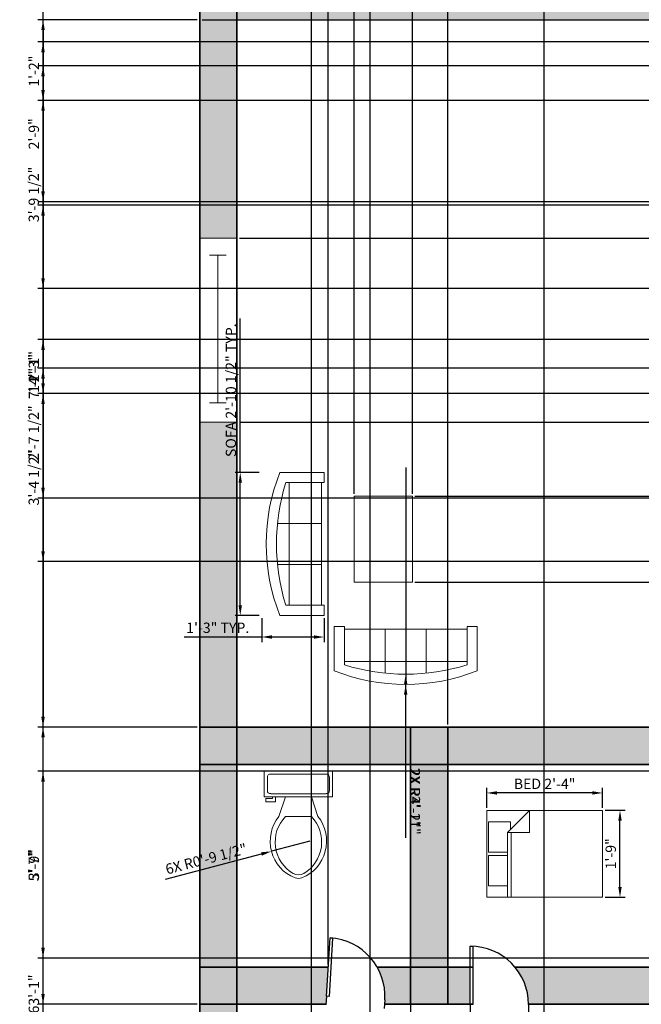
# Model space of a CAD drawing. Units: millimetres. Extents: x 2856 to 3283, y 634 to 1474.
# Tile 3 of 8: x 2856 to 3006, y 1050 to 1288. Entities that reach past the tile are written whole.
import ezdxf

# ---------------------------------------------------------------- set-up
doc = ezdxf.new("R2010")
doc.units = ezdxf.units.MM
for name, color, linetype, lineweight in [('A-ANNO-DIMS', 90, 'Continuous', 18), ('A-FLOR-FIXT', 140, 'Continuous', 18), ('A-WALL-PATT', 2, 'Continuous', 13), ('doors', 10, 'Continuous', 25), ('furniture', 140, 'Continuous', 18), ('walls', 50, 'Continuous', 35), ('windows', 30, 'Continuous', 18)]:
    doc.layers.add(name, color=color, linetype=linetype, lineweight=lineweight)
doc.styles.get("Standard").update_dxf_attribs({"font": 'arial.ttf'})
doc.dimstyles.new('ISO-25', dxfattribs={"dimtxt": 2.5, "dimasz": 2.5, "dimexe": 1.25, "dimexo": 0.625, "dimtad": 1, "dimdec": 0, "dimlunit": 3, "dimtxsty": 'Standard', "dimcen": 2.5, "dimadec": 0, "dimazin": 0, "dimtfac": 1, "dimtdec": 0, "dimtmove": 0, "dimatfit": 3, "dimfxl": 1, "dimarcsym": 0})

# ---------------------------------------------------------------- blocks, each defined once
blk = doc.blocks.new('*U3')
for p, q in [((0, 0), (0, -6)), ((40, 0), (40, -6))]:
    blk.add_line(p, q)
blk.add_lwpolyline([(0, 0), (0, 40), (1.75, 40), (1.75, 0)], close=True)
blk.add_arc((0, 0), 40, 0, 90)
blk = doc.blocks.new('*U5')
for p, q in [((0, 4), (0, 0)), ((36, 4), (36, 0)), ((0, 2), (36, 2))]:
    blk.add_line(p, q)
blk = doc.blocks.new('Bed - Queen')
for p, q in [((0, -80.00003), (0, 0)), ((0, 0), (59.99999, 0)), ((59.99999, 0), (59.99999, -80.00003)), ((7.99999, -1.2), (28.79998, -1.2)), ((7.99999, -14.4), (7.99999, -1.2)), ((28.79998, -1.2), (28.79998, -14.4)), ((31.19999, -1.2), (51.99999, -1.2)), ((31.19999, -14.4), (31.19999, -1.2)), ((51.99999, -1.2), (51.99999, -16.4)), ((0, -14.4), (44.8, -14.4)), ((44.8, -16.8), (0, -16.8)), ((59.99999, -29.6), (44.8, -14.4)), ((44.8, -14.4), (44.8, -29.6)), ((51.99999, -16.4), (46.79936, -16.4)), ((44.8, -29.6), (59.99999, -29.6)), ((59.99999, -80.00003), (0, -80.00003))]:
    blk.add_line(p, q)
blk = doc.blocks.new('Sofa - Roundback 7 ft.')
for p, q in [((-36.000027, -34), (-36.000027, -11.4696)), ((-12.00002, -32.4421), (-12.00003, -6.5971)), ((11.99997, -32.4421), (11.99998, -6.5971)), ((35.99998, -34), (35.99998, -11.4696)), ((-35.999844, -13.3819), (35.9998, -13.3819)), ((-36.000027, -32.4421), (35.99998, -32.4421))]:
    blk.add_line(p, q)
for points in [[(-36.000027, -34), (-42.000027, -34), (-42.000027, -8)], [(41.99998, -8), (41.99998, -34), (35.99998, -34)]]:
    blk.add_lwpolyline(points)
for centre, radius, start, end in [((0, -114.25), 114.25, 68.43141, 111.5686), ((-0.00001, -127.1968), 121.1968, 72.72033, 107.2797)]:
    blk.add_arc(centre, radius, start, end)
blk = doc.blocks.new('Toilet - top')
for p, q in [((9.5, -6), (9.5, -2)), ((-10, -8.5), (-8, -8.5)), ((-10, -9.5), (-10, -8.5)), ((-8, -8.5), (-8, -8)), ((-7, -8), (-7, -9.5)), ((-4, -8), (-6, -14)), ((4, -8), (6, -14)), ((-7, -9.5), (-10, -9.5)), ((4, -14), (-4, -14))]:
    blk.add_line(p, q)
blk.add_lwpolyline([(10.5, -8), (10.5, 0), (-10.5, 0), (-10.5, -8)], close=True)
for points in [[(-9.5, -2), (-9.5, -6)], [(8.5, -1), (-8.5, -1)], [(-8.5, -7), (8.5, -7)]]:
    blk.add_lwpolyline(points)
for centre, radius, start, end in [((-8.62, -1.88), 0.884, 81.8699, 188.1301), ((8.62, -1.88), 0.884, 351.8699, 98.1301), ((-8.62, -6.12), 0.884, 171.8699, 278.1301), ((8.62, -6.12), 0.884, 261.8699, 8.1301), ((3.52, -21.58), 12.17, 141.4691, 247.9714), ((4.2, -21.82), 11.33, 136.3677, 238.9468), ((-3.52, -21.58), 12.17, 292.0284, 38.5307), ((-4.2, -21.82), 11.33, 301.053, 43.6321), ((0, -27.88), 4, 245.7318, 294.2682), ((0, -29), 4, 254.8605, 285.1395)]:
    blk.add_arc(centre, radius, start, end)
blk = doc.blocks.new('*D18')
at = {"layer": 'A-ANNO-DIMS', "color": 0, "lineweight": -2, "transparency": 16777216}
for p, q in [((2968.55, 1097.45), (2968.55, 1102.28)), ((2996.57, 1097.45), (2996.57, 1102.28)), ((2994.07, 1101.03), (2971.05, 1101.03))]:
    blk.add_line(p, q, dxfattribs=at)
at = {"layer": 'A-ANNO-DIMS', "color": 0, "transparency": 16777216}
for points in [[(2971.05, 1101.45), (2971.05, 1100.62), (2968.55, 1101.03)], [(2994.07, 1101.45), (2994.07, 1100.62), (2996.57, 1101.03)]]:
    blk.add_solid(points, dxfattribs=at)
at = {"layer": 'Defpoints', "color": 0, "transparency": 16777216}
for p in [(2968.55, 1101.03), (2968.55, 1096.83), (2996.57, 1096.83)]:
    blk.add_point(p, dxfattribs=at)
at = {"layer": 'A-ANNO-DIMS', "color": 0, "transparency": 16777216, "insert": (2982.56, 1102.91), "char_height": 2.5, "attachment_point": 5}
blk.add_mtext('BED 2\'-4"', dxfattribs=at)
blk = doc.blocks.new('*D19')
at = {"layer": 'A-ANNO-DIMS', "color": 0, "lineweight": -2, "transparency": 16777216}
for p, q in [((2997.2, 1096.83), (3002.03, 1096.83)), ((3000.78, 1078.31), (3000.78, 1094.33)), ((2997.2, 1075.81), (3002.03, 1075.81))]:
    blk.add_line(p, q, dxfattribs=at)
at = {"layer": 'A-ANNO-DIMS', "color": 0, "transparency": 16777216}
for points in [[(3000.36, 1094.33), (3001.19, 1094.33), (3000.78, 1096.83)], [(3000.36, 1078.31), (3001.19, 1078.31), (3000.78, 1075.81)]]:
    blk.add_solid(points, dxfattribs=at)
at = {"layer": 'Defpoints', "color": 0, "transparency": 16777216}
for p in [(2996.57, 1096.83), (3000.78, 1096.83), (2996.57, 1075.81)]:
    blk.add_point(p, dxfattribs=at)
at = {"layer": 'A-ANNO-DIMS', "color": 0, "transparency": 16777216, "insert": (2998.87, 1086.32), "char_height": 2.5, "attachment_point": 5, "rotation": 90}
blk.add_mtext('1\'-9"', dxfattribs=at)
blk = doc.blocks.new('*D22')
at = {"layer": 'A-ANNO-DIMS', "color": 0, "lineweight": -2, "transparency": 16777216}
for p, q in [((2908.97, 1178.52), (2908.97, 1215.74)), ((2913.54, 1178.52), (2907.72, 1178.52)), ((2908.97, 1146.41), (2908.97, 1176.02)), ((2913.54, 1143.91), (2907.72, 1143.91))]:
    blk.add_line(p, q, dxfattribs=at)
at = {"layer": 'A-ANNO-DIMS', "color": 0, "transparency": 16777216}
for points in [[(2908.56, 1176.02), (2909.39, 1176.02), (2908.97, 1178.52)], [(2908.56, 1146.41), (2909.39, 1146.41), (2908.97, 1143.91)]]:
    blk.add_solid(points, dxfattribs=at)
at = {"layer": 'Defpoints', "color": 0, "transparency": 16777216}
for p in [(2908.97, 1178.52), (2914.16, 1178.52), (2914.16, 1143.91)]:
    blk.add_point(p, dxfattribs=at)
at = {"layer": 'A-ANNO-DIMS', "color": 0, "transparency": 16777216, "insert": (2907.05, 1198.38), "char_height": 2.5, "attachment_point": 5, "rotation": 90}
blk.add_mtext('SOFA 2\'-10 1/2" TYP.', dxfattribs=at)
blk = doc.blocks.new('*D23')
at = {"layer": 'A-ANNO-DIMS', "color": 0, "lineweight": -2, "transparency": 16777216}
for p, q in [((2914.16, 1143.29), (2914.16, 1137.47)), ((2929.27, 1143.29), (2929.27, 1137.47)), ((2914.16, 1138.72), (2895.41, 1138.72)), ((2926.77, 1138.72), (2916.66, 1138.72))]:
    blk.add_line(p, q, dxfattribs=at)
at = {"layer": 'A-ANNO-DIMS', "color": 0, "transparency": 16777216}
for points in [[(2916.66, 1139.14), (2916.66, 1138.31), (2914.16, 1138.72)], [(2926.77, 1139.14), (2926.77, 1138.31), (2929.27, 1138.72)]]:
    blk.add_solid(points, dxfattribs=at)
at = {"layer": 'Defpoints', "color": 0, "transparency": 16777216}
for p in [(2914.16, 1143.91), (2929.27, 1143.91), (2914.16, 1138.72)]:
    blk.add_point(p, dxfattribs=at)
at = {"layer": 'A-ANNO-DIMS', "color": 0, "transparency": 16777216, "insert": (2903.54, 1140.63), "char_height": 2.5, "attachment_point": 5}
blk.add_mtext('1\'-3" TYP.', dxfattribs=at)
blk = doc.blocks.new('*D29')
at = {"layer": 'A-ANNO-DIMS', "color": 0, "lineweight": -2, "transparency": 16777216}
for p, q in [((2898.55, 1430.94), (2860.05, 1430.94)), ((2861.3, 676.44), (2861.3, 1428.44)), ((2898.55, 673.94), (2860.05, 673.94))]:
    blk.add_line(p, q, dxfattribs=at)
at = {"layer": 'A-ANNO-DIMS', "color": 0, "transparency": 16777216}
for points in [[(2860.88, 1428.44), (2861.72, 1428.44), (2861.3, 1430.94)], [(2860.88, 676.44), (2861.72, 676.44), (2861.3, 673.94)]]:
    blk.add_solid(points, dxfattribs=at)
at = {"layer": 'Defpoints', "color": 0, "transparency": 16777216}
for p in [(2861.3, 1430.94), (2899.17, 1430.94), (2899.17, 673.94)]:
    blk.add_point(p, dxfattribs=at)
at = {"layer": 'A-ANNO-DIMS', "color": 0, "transparency": 16777216, "insert": (2859.4, 1052.44), "char_height": 2.5, "attachment_point": 5, "rotation": 90}
blk.add_mtext('63\'-1"', dxfattribs=at)
blk = doc.blocks.new('*D49')
at = {"layer": 'A-ANNO-DIMS', "color": 0, "lineweight": -2, "transparency": 16777216}
for p, q in [((2898.55, 1287.94), (2860.05, 1287.94)), ((2861.3, 1285.44), (2861.3, 1119.44)), ((2898.55, 1116.94), (2860.05, 1116.94))]:
    blk.add_line(p, q, dxfattribs=at)
at = {"layer": 'A-ANNO-DIMS', "color": 0, "transparency": 16777216}
for points in [[(2860.88, 1285.44), (2861.72, 1285.44), (2861.3, 1287.94)], [(2860.88, 1119.44), (2861.72, 1119.44), (2861.3, 1116.94)]]:
    blk.add_solid(points, dxfattribs=at)
at = {"layer": 'Defpoints', "color": 0, "transparency": 16777216}
for p in [(2899.17, 1287.94), (2861.3, 1116.94), (2899.17, 1116.94)]:
    blk.add_point(p, dxfattribs=at)
at = {"layer": 'A-ANNO-DIMS', "color": 0, "transparency": 16777216, "insert": (2859.4, 1202.44), "char_height": 2.5, "attachment_point": 5, "rotation": 90}
blk.add_mtext('14\'-3"', dxfattribs=at)
blk = doc.blocks.new('*D56')
at = {"layer": 'A-ANNO-DIMS', "color": 0, "lineweight": -2, "transparency": 16777216}
for p, q in [((3105.44, 1106.29), (2860.05, 1106.29)), ((2861.3, 1063.61), (2861.3, 1103.79)), ((3105.89, 1061.11), (2860.05, 1061.11))]:
    blk.add_line(p, q, dxfattribs=at)
at = {"layer": 'A-ANNO-DIMS', "color": 0, "transparency": 16777216}
for points in [[(2860.88, 1103.79), (2861.72, 1103.79), (2861.3, 1106.29)], [(2860.88, 1063.61), (2861.72, 1063.61), (2861.3, 1061.11)]]:
    blk.add_solid(points, dxfattribs=at)
at = {"layer": 'Defpoints', "color": 0, "transparency": 16777216}
for p in [(2861.3, 1106.29), (3106.06, 1106.29), (3106.52, 1061.11)]:
    blk.add_point(p, dxfattribs=at)
at = {"layer": 'A-ANNO-DIMS', "color": 0, "transparency": 16777216, "insert": (2859.4, 1083.7), "char_height": 2.5, "attachment_point": 5, "rotation": 90}
blk.add_mtext('3\'-9"', dxfattribs=at)
blk = doc.blocks.new('*D58')
at = {"layer": 'A-ANNO-DIMS', "color": 0, "lineweight": -2, "transparency": 16777216}
for p, q in [((2950.17, 1116.31), (2950.17, 634.81)), ((2899.17, 1107.31), (2899.17, 634.81)), ((2901.67, 636.06), (2947.67, 636.06))]:
    blk.add_line(p, q, dxfattribs=at)
at = {"layer": 'A-ANNO-DIMS', "color": 0, "transparency": 16777216}
for points in [[(2901.67, 636.48), (2901.67, 635.65), (2899.17, 636.06)], [(2947.67, 636.48), (2947.67, 635.65), (2950.17, 636.06)]]:
    blk.add_solid(points, dxfattribs=at)
at = {"layer": 'Defpoints', "color": 0, "transparency": 16777216}
for p in [(2950.17, 1116.94), (2899.17, 1107.94), (2950.17, 636.06)]:
    blk.add_point(p, dxfattribs=at)
at = {"layer": 'A-ANNO-DIMS', "color": 0, "transparency": 16777216, "insert": (2924.67, 637.97), "char_height": 2.5, "attachment_point": 5}
blk.add_mtext('4\'-3"', dxfattribs=at)
blk = doc.blocks.new('*D59')
at = {"layer": 'A-ANNO-DIMS', "color": 0, "lineweight": -2, "transparency": 16777216}
for p, q in [((2959.17, 1117.56), (2959.17, 1470.06)), ((2961.67, 1468.81), (3071.67, 1468.81)), ((3074.17, 1117.56), (3074.17, 1470.06))]:
    blk.add_line(p, q, dxfattribs=at)
at = {"layer": 'A-ANNO-DIMS', "color": 0, "transparency": 16777216}
for points in [[(2961.67, 1469.23), (2961.67, 1468.4), (2959.17, 1468.81)], [(3071.67, 1469.23), (3071.67, 1468.4), (3074.17, 1468.81)]]:
    blk.add_solid(points, dxfattribs=at)
at = {"layer": 'Defpoints', "color": 0, "transparency": 16777216}
for p in [(3074.17, 1468.81), (2959.17, 1116.94), (3074.17, 1116.94)]:
    blk.add_point(p, dxfattribs=at)
at = {"layer": 'A-ANNO-DIMS', "color": 0, "transparency": 16777216, "insert": (3016.67, 1470.71), "char_height": 2.5, "attachment_point": 5}
blk.add_mtext('9\'-7"', dxfattribs=at)
blk = doc.blocks.new('*D60')
at = {"layer": 'A-ANNO-DIMS', "color": 0, "lineweight": -2, "transparency": 16777216}
for p, q in [((2898.55, 1116.94), (2860.05, 1116.94)), ((2861.3, 1052.44), (2861.3, 1114.44)), ((2898.55, 1049.94), (2860.05, 1049.94))]:
    blk.add_line(p, q, dxfattribs=at)
at = {"layer": 'A-ANNO-DIMS', "color": 0, "transparency": 16777216}
for points in [[(2860.88, 1114.44), (2861.72, 1114.44), (2861.3, 1116.94)], [(2860.88, 1052.44), (2861.72, 1052.44), (2861.3, 1049.94)]]:
    blk.add_solid(points, dxfattribs=at)
at = {"layer": 'Defpoints', "color": 0, "transparency": 16777216}
for p in [(2861.3, 1116.94), (2899.17, 1116.94), (2899.17, 1049.94)]:
    blk.add_point(p, dxfattribs=at)
at = {"layer": 'A-ANNO-DIMS', "color": 0, "transparency": 16777216, "insert": (2859.4, 1083.44), "char_height": 2.5, "attachment_point": 5, "rotation": 90}
blk.add_mtext('5\'-7"', dxfattribs=at)
blk = doc.blocks.new('*D63')
at = {"layer": 'A-ANNO-DIMS', "color": 0, "lineweight": -2, "transparency": 16777216}
for p, q in [((3164.55, 1282.56), (2860.05, 1282.56)), ((2861.3, 1270.93), (2861.3, 1280.06)), ((3164.55, 1268.43), (2860.05, 1268.43))]:
    blk.add_line(p, q, dxfattribs=at)
at = {"layer": 'A-ANNO-DIMS', "color": 0, "transparency": 16777216}
for points in [[(2860.88, 1280.06), (2861.72, 1280.06), (2861.3, 1282.56)], [(2860.88, 1270.93), (2861.72, 1270.93), (2861.3, 1268.43)]]:
    blk.add_solid(points, dxfattribs=at)
at = {"layer": 'Defpoints', "color": 0, "transparency": 16777216}
for p in [(2861.3, 1282.56), (3165.17, 1282.56), (3165.17, 1268.43)]:
    blk.add_point(p, dxfattribs=at)
at = {"layer": 'A-ANNO-DIMS', "color": 0, "transparency": 16777216, "insert": (2859.42, 1275.5), "char_height": 2.5, "attachment_point": 5, "rotation": 90}
blk.add_mtext('1\'-2"', dxfattribs=at)
blk = doc.blocks.new('*D64')
at = {"layer": 'A-ANNO-DIMS', "color": 0, "lineweight": -2, "transparency": 16777216}
for p, q in [((3164.55, 1210.62), (2860.05, 1210.62)), ((2861.3, 1200.05), (2861.3, 1208.12)), ((3164.55, 1197.55), (2860.05, 1197.55))]:
    blk.add_line(p, q, dxfattribs=at)
at = {"layer": 'A-ANNO-DIMS', "color": 0, "transparency": 16777216}
for points in [[(2860.88, 1208.12), (2861.72, 1208.12), (2861.3, 1210.62)], [(2860.88, 1200.05), (2861.72, 1200.05), (2861.3, 1197.55)]]:
    blk.add_solid(points, dxfattribs=at)
at = {"layer": 'Defpoints', "color": 0, "transparency": 16777216}
for p in [(2861.3, 1210.62), (3165.17, 1210.62), (3165.17, 1197.55)]:
    blk.add_point(p, dxfattribs=at)
at = {"layer": 'A-ANNO-DIMS', "color": 0, "transparency": 16777216, "insert": (2859.42, 1204.09), "char_height": 2.5, "attachment_point": 5, "rotation": 90}
blk.add_mtext('1\'-1"', dxfattribs=at)
blk = doc.blocks.new('*D69')
at = {"layer": 'A-ANNO-DIMS', "color": 0, "lineweight": -2, "transparency": 16777216}
for p, q in [((2940.27, 1421.31), (2940.27, 634.81)), ((2982.35, 1421.31), (2982.35, 634.81)), ((2942.77, 636.06), (2979.85, 636.06))]:
    blk.add_line(p, q, dxfattribs=at)
at = {"layer": 'A-ANNO-DIMS', "color": 0, "transparency": 16777216}
for points in [[(2942.77, 636.48), (2942.77, 635.65), (2940.27, 636.06)], [(2979.85, 636.48), (2979.85, 635.65), (2982.35, 636.06)]]:
    blk.add_solid(points, dxfattribs=at)
at = {"layer": 'Defpoints', "color": 0, "transparency": 16777216}
for p in [(2940.27, 1421.94), (2982.35, 1421.94), (2982.35, 636.06)]:
    blk.add_point(p, dxfattribs=at)
at = {"layer": 'A-ANNO-DIMS', "color": 0, "transparency": 16777216, "insert": (2961.31, 637.97), "char_height": 2.5, "attachment_point": 5}
blk.add_mtext('3\'-6"', dxfattribs=at)
blk = doc.blocks.new('*D73')
at = {"layer": 'A-ANNO-DIMS', "color": 0, "lineweight": -2, "transparency": 16777216}
for p, q in [((2908.8, 1235.12), (3282.3, 1235.12)), ((3281.05, 1193.19), (3281.05, 1232.62)), ((2908.8, 1190.69), (3282.3, 1190.69))]:
    blk.add_line(p, q, dxfattribs=at)
at = {"layer": 'A-ANNO-DIMS', "color": 0, "transparency": 16777216}
for points in [[(3280.63, 1232.62), (3281.47, 1232.62), (3281.05, 1235.12)], [(3280.63, 1193.19), (3281.47, 1193.19), (3281.05, 1190.69)]]:
    blk.add_solid(points, dxfattribs=at)
at = {"layer": 'Defpoints', "color": 0, "transparency": 16777216}
for p in [(2908.17, 1235.12), (3281.05, 1235.12), (2908.17, 1190.69)]:
    blk.add_point(p, dxfattribs=at)
at = {"layer": 'A-ANNO-DIMS', "color": 0, "transparency": 16777216, "insert": (3279.13, 1212.91), "char_height": 2.5, "attachment_point": 5, "rotation": 90}
blk.add_mtext('3\'-8 1/2"', dxfattribs=at)
blk = doc.blocks.new('*D74')
at = {"layer": 'A-ANNO-DIMS', "color": 0, "lineweight": -2, "transparency": 16777216}
for p, q in [((3233.55, 1276.76), (2860.05, 1276.76)), ((2861.3, 1246.44), (2861.3, 1274.26)), ((3233.55, 1243.94), (2860.05, 1243.94))]:
    blk.add_line(p, q, dxfattribs=at)
at = {"layer": 'A-ANNO-DIMS', "color": 0, "transparency": 16777216}
for points in [[(2860.88, 1274.26), (2861.72, 1274.26), (2861.3, 1276.76)], [(2860.88, 1246.44), (2861.72, 1246.44), (2861.3, 1243.94)]]:
    blk.add_solid(points, dxfattribs=at)
at = {"layer": 'Defpoints', "color": 0, "transparency": 16777216}
for p in [(2861.3, 1276.76), (3234.17, 1276.76), (3234.17, 1243.94)]:
    blk.add_point(p, dxfattribs=at)
at = {"layer": 'A-ANNO-DIMS', "color": 0, "transparency": 16777216, "insert": (2859.4, 1260.35), "char_height": 2.5, "attachment_point": 5, "rotation": 90}
blk.add_mtext('2\'-9"', dxfattribs=at)
blk = doc.blocks.new('*D75')
at = {"layer": 'A-ANNO-DIMS', "color": 0, "lineweight": -2, "transparency": 16777216}
for p, q in [((3233.55, 1203.68), (2860.05, 1203.68)), ((2861.3, 1174.81), (2861.3, 1201.18)), ((3233.55, 1172.31), (2860.05, 1172.31))]:
    blk.add_line(p, q, dxfattribs=at)
at = {"layer": 'A-ANNO-DIMS', "color": 0, "transparency": 16777216}
for points in [[(2860.88, 1201.18), (2861.72, 1201.18), (2861.3, 1203.68)], [(2860.88, 1174.81), (2861.72, 1174.81), (2861.3, 1172.31)]]:
    blk.add_solid(points, dxfattribs=at)
at = {"layer": 'Defpoints', "color": 0, "transparency": 16777216}
for p in [(2861.3, 1203.68), (3234.17, 1203.68), (3234.17, 1172.31)]:
    blk.add_point(p, dxfattribs=at)
at = {"layer": 'A-ANNO-DIMS', "color": 0, "transparency": 16777216, "insert": (2859.38, 1188), "char_height": 2.5, "attachment_point": 5, "rotation": 90}
blk.add_mtext('2\'-7 1/2"', dxfattribs=at)
blk = doc.blocks.new('*D76')
at = {"layer": 'A-ANNO-DIMS', "color": 0, "lineweight": -2, "transparency": 16777216}
for p, q in [((2899.17, 1421.31), (2899.17, 634.81)), ((2940.27, 1421.31), (2940.27, 634.81)), ((2901.67, 636.06), (2937.77, 636.06))]:
    blk.add_line(p, q, dxfattribs=at)
at = {"layer": 'A-ANNO-DIMS', "color": 0, "transparency": 16777216}
for points in [[(2901.67, 636.48), (2901.67, 635.65), (2899.17, 636.06)], [(2937.77, 636.48), (2937.77, 635.65), (2940.27, 636.06)]]:
    blk.add_solid(points, dxfattribs=at)
at = {"layer": 'Defpoints', "color": 0, "transparency": 16777216}
for p in [(2899.17, 1421.94), (2940.27, 1421.94), (2940.27, 636.06)]:
    blk.add_point(p, dxfattribs=at)
at = {"layer": 'A-ANNO-DIMS', "color": 0, "transparency": 16777216, "insert": (2919.72, 637.97), "char_height": 2.5, "attachment_point": 5}
blk.add_mtext('3\'-5"', dxfattribs=at)
blk = doc.blocks.new('*D79')
at = {"layer": 'A-ANNO-DIMS', "color": 0, "lineweight": -2, "transparency": 16777216}
for p, q in [((2899.8, 1287.94), (3282.3, 1287.94)), ((3281.05, 1237.62), (3281.05, 1285.44)), ((2908.8, 1235.12), (3282.3, 1235.12))]:
    blk.add_line(p, q, dxfattribs=at)
at = {"layer": 'A-ANNO-DIMS', "color": 0, "transparency": 16777216}
for points in [[(3280.63, 1285.44), (3281.47, 1285.44), (3281.05, 1287.94)], [(3280.63, 1237.62), (3281.47, 1237.62), (3281.05, 1235.12)]]:
    blk.add_solid(points, dxfattribs=at)
at = {"layer": 'Defpoints', "color": 0, "transparency": 16777216}
for p in [(2899.17, 1287.94), (3281.05, 1287.94), (2908.17, 1235.12)]:
    blk.add_point(p, dxfattribs=at)
at = {"layer": 'A-ANNO-DIMS', "color": 0, "transparency": 16777216, "insert": (3279.15, 1261.53), "char_height": 2.5, "attachment_point": 5, "rotation": 90}
blk.add_mtext('4\'-5"', dxfattribs=at)
blk = doc.blocks.new('*D82')
at = {"layer": 'A-ANNO-DIMS', "color": 0, "lineweight": -2, "transparency": 16777216}
for p, q in [((2936.5, 1173.36), (2936.5, 1470.06)), ((2939, 1468.81), (2948.08, 1468.81)), ((2950.58, 1173.36), (2950.58, 1470.06))]:
    blk.add_line(p, q, dxfattribs=at)
at = {"layer": 'A-ANNO-DIMS', "color": 0, "transparency": 16777216}
for points in [[(2939, 1469.23), (2939, 1468.4), (2936.5, 1468.81)], [(2948.08, 1469.23), (2948.08, 1468.4), (2950.58, 1468.81)]]:
    blk.add_solid(points, dxfattribs=at)
at = {"layer": 'Defpoints', "color": 0, "transparency": 16777216}
for p in [(2950.58, 1468.81), (2936.5, 1172.73), (2950.58, 1172.73)]:
    blk.add_point(p, dxfattribs=at)
at = {"layer": 'A-ANNO-DIMS', "color": 0, "transparency": 16777216, "insert": (2943.54, 1470.69), "char_height": 2.5, "attachment_point": 5}
blk.add_mtext('1\'-2"', dxfattribs=at)
blk = doc.blocks.new('*D83')
at = {"layer": 'A-ANNO-DIMS', "color": 0, "lineweight": -2, "transparency": 16777216}
for p, q in [((2951.21, 1172.73), (3282.3, 1172.73)), ((3281.05, 1154.47), (3281.05, 1170.23)), ((2951.21, 1151.97), (3282.3, 1151.97))]:
    blk.add_line(p, q, dxfattribs=at)
at = {"layer": 'A-ANNO-DIMS', "color": 0, "transparency": 16777216}
for points in [[(3280.63, 1170.23), (3281.47, 1170.23), (3281.05, 1172.73)], [(3280.63, 1154.47), (3281.47, 1154.47), (3281.05, 1151.97)]]:
    blk.add_solid(points, dxfattribs=at)
at = {"layer": 'Defpoints', "color": 0, "transparency": 16777216}
for p in [(2950.58, 1172.73), (3281.05, 1172.73), (2950.58, 1151.97)]:
    blk.add_point(p, dxfattribs=at)
at = {"layer": 'A-ANNO-DIMS', "color": 0, "transparency": 16777216, "insert": (3279.15, 1162.35), "char_height": 2.5, "attachment_point": 5, "rotation": 90}
blk.add_mtext('1\'-9"', dxfattribs=at)
blk = doc.blocks.new('*D84')
at = {"layer": 'A-ANNO-DIMS', "color": 0, "lineweight": -2, "transparency": 16777216}
for p, q in [((3164.55, 1268.43), (2860.05, 1268.43)), ((2861.3, 1225.44), (2861.3, 1265.93)), ((3164.55, 1222.94), (2860.05, 1222.94))]:
    blk.add_line(p, q, dxfattribs=at)
at = {"layer": 'A-ANNO-DIMS', "color": 0, "transparency": 16777216}
for points in [[(2860.88, 1265.93), (2861.72, 1265.93), (2861.3, 1268.43)], [(2860.88, 1225.44), (2861.72, 1225.44), (2861.3, 1222.94)]]:
    blk.add_solid(points, dxfattribs=at)
at = {"layer": 'Defpoints', "color": 0, "transparency": 16777216}
for p in [(2861.3, 1268.43), (3165.17, 1268.43), (3165.17, 1222.94)]:
    blk.add_point(p, dxfattribs=at)
at = {"layer": 'A-ANNO-DIMS', "color": 0, "transparency": 16777216, "insert": (2859.38, 1245.69), "char_height": 2.5, "attachment_point": 5, "rotation": 90}
blk.add_mtext('3\'-9 1/2"', dxfattribs=at)
blk = doc.blocks.new('*D85')
at = {"layer": 'A-ANNO-DIMS', "color": 0, "lineweight": -2, "transparency": 16777216}
for p, q in [((3164.55, 1197.55), (2860.05, 1197.55)), ((2861.3, 1159.44), (2861.3, 1195.05)), ((3164.55, 1156.94), (2860.05, 1156.94))]:
    blk.add_line(p, q, dxfattribs=at)
at = {"layer": 'A-ANNO-DIMS', "color": 0, "transparency": 16777216}
for points in [[(2860.88, 1195.05), (2861.72, 1195.05), (2861.3, 1197.55)], [(2860.88, 1159.44), (2861.72, 1159.44), (2861.3, 1156.94)]]:
    blk.add_solid(points, dxfattribs=at)
at = {"layer": 'Defpoints', "color": 0, "transparency": 16777216}
for p in [(2861.3, 1197.55), (3165.17, 1197.55), (3165.17, 1156.94)]:
    blk.add_point(p, dxfattribs=at)
at = {"layer": 'A-ANNO-DIMS', "color": 0, "transparency": 16777216, "insert": (2859.38, 1177.24), "char_height": 2.5, "attachment_point": 5, "rotation": 90}
blk.add_mtext('3\'-4 1/2"', dxfattribs=at)
blk = doc.blocks.new('*D86')
at = {"layer": 'A-ANNO-DIMS', "color": 0, "lineweight": -2, "transparency": 16777216}
for p, q in [((2899.17, 1059.56), (2899.17, 1470.06)), ((2901.67, 1468.81), (2927.75, 1468.81)), ((2930.25, 1059.56), (2930.25, 1470.06))]:
    blk.add_line(p, q, dxfattribs=at)
at = {"layer": 'A-ANNO-DIMS', "color": 0, "transparency": 16777216}
for points in [[(2901.67, 1469.23), (2901.67, 1468.4), (2899.17, 1468.81)], [(2927.75, 1469.23), (2927.75, 1468.4), (2930.25, 1468.81)]]:
    blk.add_solid(points, dxfattribs=at)
at = {"layer": 'Defpoints', "color": 0, "transparency": 16777216}
for p in [(2930.25, 1468.81), (2899.17, 1058.94), (2930.25, 1058.94)]:
    blk.add_point(p, dxfattribs=at)
at = {"layer": 'A-ANNO-DIMS', "color": 0, "transparency": 16777216, "insert": (2914.71, 1470.69), "char_height": 2.5, "attachment_point": 5}
blk.add_mtext('2\'-7"', dxfattribs=at)
blk = doc.blocks.new('*D90')
at = {"layer": 'A-ANNO-DIMS', "color": 0, "lineweight": -2, "transparency": 16777216}
for p, q in [((2899.17, 1421.31), (2899.17, 634.81)), ((2926.08, 1404.73), (2926.08, 634.81)), ((2901.67, 636.06), (2923.58, 636.06))]:
    blk.add_line(p, q, dxfattribs=at)
at = {"layer": 'A-ANNO-DIMS', "color": 0, "transparency": 16777216}
for points in [[(2901.67, 636.48), (2901.67, 635.65), (2899.17, 636.06)], [(2923.58, 636.48), (2923.58, 635.65), (2926.08, 636.06)]]:
    blk.add_solid(points, dxfattribs=at)
at = {"layer": 'Defpoints', "color": 0, "transparency": 16777216}
for p in [(2899.17, 1421.94), (2926.08, 1405.35), (2926.08, 636.06)]:
    blk.add_point(p, dxfattribs=at)
at = {"layer": 'A-ANNO-DIMS', "color": 0, "transparency": 16777216, "insert": (2912.63, 637.97), "char_height": 2.5, "attachment_point": 5}
blk.add_mtext('2\'-3"', dxfattribs=at)
blk = doc.blocks.new('*D95')
at = {"layer": 'A-ANNO-DIMS', "color": 0, "lineweight": -2, "transparency": 16777216}
for p, q in [((3108.57, 1243.09), (2860.05, 1243.09)), ((2861.3, 1159.44), (2861.3, 1240.59)), ((3164.55, 1156.94), (2860.05, 1156.94))]:
    blk.add_line(p, q, dxfattribs=at)
at = {"layer": 'A-ANNO-DIMS', "color": 0, "transparency": 16777216}
for points in [[(2860.88, 1240.59), (2861.72, 1240.59), (2861.3, 1243.09)], [(2860.88, 1159.44), (2861.72, 1159.44), (2861.3, 1156.94)]]:
    blk.add_solid(points, dxfattribs=at)
at = {"layer": 'Defpoints', "color": 0, "transparency": 16777216}
for p in [(2861.3, 1243.09), (3109.2, 1243.09), (3165.17, 1156.94)]:
    blk.add_point(p, dxfattribs=at)
at = {"layer": 'A-ANNO-DIMS', "color": 0, "transparency": 16777216, "insert": (2859.42, 1200.02), "char_height": 2.5, "attachment_point": 5, "rotation": 90}
blk.add_mtext('7\'-2"', dxfattribs=at)
blk = doc.blocks.new('*D99')
at = {"layer": 'A-ANNO-DIMS', "color": 0, "lineweight": -2, "transparency": 16777216}
for p, q in [((2948.97, 1179.66), (2948.97, 1129.73)), ((2948.97, 1091.93), (2948.97, 1127.23))]:
    blk.add_line(p, q, dxfattribs=at)
at = {"layer": 'A-ANNO-DIMS', "color": 0, "transparency": 16777216}
blk.add_solid([(2949.39, 1127.23), (2948.55, 1127.23), (2948.97, 1129.73)], dxfattribs=at)
at = {"layer": 'Defpoints', "color": 0, "transparency": 16777216}
for p in [(2948.97, 1179.66), (2948.97, 1129.73)]:
    blk.add_point(p, dxfattribs=at)
at = {"layer": 'A-ANNO-DIMS', "color": 0, "transparency": 16777216, "insert": (2950.85, 1099.78), "char_height": 2.5, "attachment_point": 5, "rotation": 270.0006}
blk.add_mtext('2X R4\'-2"', dxfattribs=at)
blk = doc.blocks.new('*D100')
at = {"layer": 'A-ANNO-DIMS', "color": 0, "lineweight": -2, "transparency": 16777216}
for p, q in [((2948.97, 1174.33), (2948.97, 1127.26)), ((2948.97, 1090.2), (2948.97, 1124.76))]:
    blk.add_line(p, q, dxfattribs=at)
at = {"layer": 'A-ANNO-DIMS', "color": 0, "transparency": 16777216}
blk.add_solid([(2949.39, 1124.76), (2948.55, 1124.76), (2948.97, 1127.26)], dxfattribs=at)
at = {"layer": 'Defpoints', "color": 0, "transparency": 16777216}
for p in [(2948.97, 1174.33), (2948.97, 1127.26)]:
    blk.add_point(p, dxfattribs=at)
at = {"layer": 'A-ANNO-DIMS', "color": 0, "transparency": 16777216, "insert": (2950.87, 1099.02), "char_height": 2.5, "attachment_point": 5, "rotation": 270.0006}
blk.add_mtext('2X R3\'-11"', dxfattribs=at)
blk = doc.blocks.new('*D101')
at = {"layer": 'A-ANNO-DIMS', "color": 0, "lineweight": -2, "transparency": 16777216}
for p, q in [((2925.81, 1089.36), (2916.54, 1086.92)), ((2890.91, 1080.18), (2914.12, 1086.29))]:
    blk.add_line(p, q, dxfattribs=at)
at = {"layer": 'A-ANNO-DIMS', "color": 0, "transparency": 16777216}
blk.add_solid([(2914.01, 1086.69), (2914.22, 1085.88), (2916.54, 1086.92)], dxfattribs=at)
at = {"layer": 'Defpoints', "color": 0, "transparency": 16777216}
for p in [(2925.81, 1089.36), (2916.54, 1086.92)]:
    blk.add_point(p, dxfattribs=at)
at = {"layer": 'A-ANNO-DIMS', "color": 0, "transparency": 16777216, "insert": (2900.82, 1084.77), "char_height": 2.5, "attachment_point": 5, "rotation": 14.7308}
blk.add_mtext('6X R0\'-9 1/2"', dxfattribs=at)

msp = doc.modelspace()

# ---------------------------------------------------------------- hatches: boundary and pattern name
at = {"layer": 'A-WALL-PATT'}
h = msp.add_hatch(color=256, dxfattribs=at)
h.dxf.hatch_style = 1
h.paths.add_polyline_path([(2908.17, 1430.94), (2899.17, 1430.94), (2899.17, 1421.94), (2908.17, 1421.94)])
h.paths.add_polyline_path([(2908.17, 1421.94), (2899.17, 1421.94), (2899.17, 1296.94), (2908.17, 1296.94)])
h.paths.add_polyline_path([(2940.27, 1430.94), (2908.17, 1430.94), (2908.17, 1421.94), (2940.27, 1421.94)])
h.paths.add_polyline_path([(3031.17, 1430.94), (2982.35, 1430.94), (2982.35, 1421.94), (3031.17, 1421.94)])
h.paths.add_polyline_path([(3150.5, 1430.94), (3097.17, 1430.94), (3097.17, 1421.94), (3150.5, 1421.94)])
h.paths.add_polyline_path([(3097.17, 1430.94), (3088.17, 1430.94), (3088.17, 1421.94), (3097.17, 1421.94)])
h.paths.add_polyline_path([(3097.17, 1421.94), (3088.17, 1421.94), (3088.17, 1337.94), (3097.17, 1337.94)])
h.paths.add_polyline_path([(3088.17, 1337.94), (3040.17, 1337.94), (3040.17, 1328.94), (3088.17, 1328.94)])
h.paths.add_polyline_path([(3097.17, 1337.94), (3088.17, 1337.94), (3088.17, 1328.94), (3097.17, 1328.94)])
h.paths.add_polyline_path([(3097.17, 1328.94), (3088.17, 1328.94), (3088.17, 1296.94), (3097.17, 1296.94)])
h.paths.add_polyline_path([(3097.17, 1296.94), (3088.17, 1296.94), (3088.17, 1287.94), (3097.17, 1287.94)])
h.paths.add_polyline_path([(3040.17, 1421.94), (3031.17, 1421.94), (3031.17, 1337.94), (3040.17, 1337.94)])
h.paths.add_polyline_path([(3040.17, 1337.94), (3031.17, 1337.94), (3031.17, 1328.94), (3040.17, 1328.94)])
h.paths.add_polyline_path([(3040.17, 1430.94), (3031.17, 1430.94), (3031.17, 1421.94), (3040.17, 1421.94)])
h.paths.add_polyline_path([(3243.17, 1421.94), (3234.17, 1421.94), (3234.17, 1385.21), (3243.17, 1385.21)])
h.paths.add_polyline_path([(3243.17, 1430.94), (3234.17, 1430.94), (3234.17, 1421.94), (3243.17, 1421.94)])
h.paths.add_polyline_path([(3234.17, 1430.94), (3189.65, 1430.94), (3189.65, 1421.94), (3234.17, 1421.94)])
h.paths.add_polyline_path([(3243.17, 1345.16), (3234.17, 1345.16), (3234.17, 1296.94), (3243.17, 1296.94)])
h.paths.add_polyline_path([(3234.17, 1296.94), (3128.45, 1296.94, -0.06768), (3129.44, 1289.59), (3129.44, 1287.94), (3234.17, 1287.94)])
h.paths.add_polyline_path([(3031.17, 1296.94), (2908.17, 1296.94), (2908.17, 1287.94), (3031.17, 1287.94)])
h.paths.add_polyline_path([(3040.17, 1296.94), (3031.17, 1296.94), (3031.17, 1287.94), (3040.17, 1287.94)])
h.paths.add_polyline_path([(2908.17, 1296.94), (2899.17, 1296.94), (2899.17, 1287.94), (2908.17, 1287.94)])
h.paths.add_polyline_path([(2908.17, 1287.94), (2899.17, 1287.94), (2899.17, 1235.12), (2908.17, 1235.12)])
h.paths.add_polyline_path([(3040.17, 1287.94), (3031.17, 1287.94), (3031.17, 1165.94), (3040.17, 1165.94)])
h.paths.add_polyline_path([(3165.17, 1165.94), (3040.17, 1165.94), (3040.17, 1156.94), (3165.17, 1156.94)])
h.paths.add_polyline_path([(3040.17, 1165.94), (3031.17, 1165.94), (3031.17, 1156.94), (3040.17, 1156.94)])
h.paths.add_polyline_path([(3040.17, 1156.94), (3031.17, 1156.94), (3031.17, 1147.75, -0.068303), (3038.59, 1148.77), (3040.17, 1148.77)])
h.paths.add_polyline_path([(3174.17, 1197.55), (3166.11, 1197.55), (3165.17, 1197.55), (3165.17, 1165.94), (3174.17, 1165.94)])
h.paths.add_polyline_path([(3174.17, 1165.94), (3165.17, 1165.94), (3165.17, 1156.94), (3174.17, 1156.94)])
h.paths.add_polyline_path([(3234.17, 1165.94), (3174.17, 1165.94), (3174.17, 1156.94), (3234.17, 1156.94)])
h.paths.add_polyline_path([(3243.17, 1165.94), (3234.17, 1165.94), (3234.17, 1156.94), (3243.17, 1156.94)])
h.paths.add_polyline_path([(3243.17, 1172.31), (3234.17, 1172.31), (3234.17, 1165.94), (3243.17, 1165.94)])
h.paths.add_polyline_path([(3243.17, 1222.94), (3234.17, 1222.94), (3234.17, 1213.94), (3243.17, 1213.94)])
h.paths.add_polyline_path([(3234.17, 1222.94), (3174.17, 1222.94), (3174.17, 1213.94), (3234.17, 1213.94)])
h.paths.add_polyline_path([(3174.17, 1222.94), (3165.17, 1222.94), (3165.17, 1213.94), (3174.17, 1213.94)])
h.paths.add_polyline_path([(3174.17, 1270.54, -0.139319), (3166.75, 1268.43), (3165.17, 1268.43), (3165.17, 1222.94), (3174.17, 1222.94)])
h.paths.add_polyline_path([(3243.17, 1243.94), (3234.17, 1243.94), (3234.17, 1222.94), (3243.17, 1222.94)])
h.paths.add_polyline_path([(3243.17, 1213.94), (3234.17, 1213.94), (3234.17, 1203.68), (3243.17, 1203.68)])
h.paths.add_polyline_path([(3174.17, 1213.94), (3165.17, 1213.94), (3165.17, 1210.62), (3166.11, 1210.62, -0.16772), (3174.17, 1207.84)])
h.paths.add_polyline_path([(3243.17, 1296.94), (3234.17, 1296.94), (3234.17, 1287.94), (3243.17, 1287.94)])
h.paths.add_polyline_path([(3243.17, 1287.94), (3234.17, 1287.94), (3234.17, 1276.76), (3243.17, 1276.76)])
h.paths.add_polyline_path([(3174.17, 1287.94), (3165.17, 1287.94), (3165.17, 1282.56), (3166.75, 1282.56), (3174.17, 1282.56)])
h.paths.add_polyline_path([(2908.17, 1190.69), (2899.17, 1190.69), (2899.17, 1116.94), (2908.17, 1116.94)])
h.paths.add_polyline_path([(2908.17, 1107.94), (2899.17, 1107.94), (2899.17, 1058.94), (2908.17, 1058.94)])
h.paths.add_polyline_path([(2908.17, 1116.94), (2899.17, 1116.94), (2899.17, 1107.94), (2908.17, 1107.94)])
h.paths.add_polyline_path([(2959.17, 1107.94), (2950.17, 1107.94), (2950.17, 1058.94), (2959.17, 1058.94)])
h.paths.add_polyline_path([(2959.17, 1116.94), (2950.17, 1116.94), (2950.17, 1107.94), (2959.17, 1107.94)])
h.paths.add_polyline_path([(2950.17, 1116.94), (2908.17, 1116.94), (2908.17, 1107.94), (2950.17, 1107.94)])
h.paths.add_polyline_path([(3031.17, 1116.94), (2959.17, 1116.94), (2959.17, 1107.94), (3031.17, 1107.94)])
h.paths.add_polyline_path([(3074.17, 1116.94), (3065.17, 1116.94), (3065.17, 1107.94), (3074.17, 1107.94)])
h.paths.add_polyline_path([(3065.17, 1116.94), (3040.17, 1116.94), (3040.17, 1107.94), (3065.17, 1107.94)])
h.paths.add_polyline_path([(3040.17, 1116.94), (3031.17, 1116.94), (3031.17, 1107.94), (3040.17, 1107.94)])
h.paths.add_polyline_path([(3040.17, 1121.26), (3038.59, 1121.26), (3031.17, 1121.26), (3031.17, 1116.94), (3040.17, 1116.94)])
h.paths.add_polyline_path([(3074.17, 1107.94), (3065.17, 1107.94), (3065.17, 1058.94), (3074.17, 1058.94)])
h.paths.add_polyline_path([(3074.17, 1058.94), (3065.17, 1058.94), (3065.17, 1049.94), (3074.17, 1049.94)])
h.paths.add_polyline_path([(3065.17, 1058.94), (2975.4, 1058.94, -0.174756), (2978.69, 1049.94), (3065.17, 1049.94)])
h.paths.add_polyline_path([(2929.83, 1051.89), (2930.25, 1058.94), (2908.17, 1058.94), (2908.17, 1049.94), (2929.71, 1049.94)])
h.paths.add_polyline_path([(2908.17, 1058.94), (2899.17, 1058.94), (2899.17, 1049.94), (2908.17, 1049.94)])
h.paths.add_polyline_path([(2950.17, 1058.94), (2942.07, 1058.94, -0.146602), (2943.93, 1051.05), (2943.86, 1049.94), (2950.17, 1049.94)])
h.paths.add_polyline_path([(2959.17, 1058.94), (2950.17, 1058.94), (2950.17, 1049.94), (2959.17, 1049.94)])
h.paths.add_polyline_path([(2964.56, 1058.94), (2959.17, 1058.94), (2959.17, 1049.94), (2964.56, 1049.94)])
h.paths.add_polyline_path([(2908.17, 1049.94), (2899.17, 1049.94), (2899.17, 799.94), (2908.17, 799.94)])
h.paths.add_polyline_path([(3234.17, 1058.94), (3074.17, 1058.94), (3074.17, 1049.94), (3234.17, 1049.94)])
h.paths.add_polyline_path([(3243.17, 1156.94), (3234.17, 1156.94), (3234.17, 1058.94), (3243.17, 1058.94)])
h.paths.add_polyline_path([(3243.17, 1058.94), (3234.17, 1058.94), (3234.17, 1049.94), (3243.17, 1049.94)])
h.paths.add_polyline_path([(3243.17, 1049.94), (3234.17, 1049.94), (3234.17, 931.7), (3234.17, 799.94), (3243.17, 799.94), (3243.17, 931.7)])
h.paths.add_polyline_path([(2908.17, 790.94), (2899.17, 790.94), (2899.17, 682.94), (2908.17, 682.94)])
h.paths.add_polyline_path([(2908.17, 799.94), (2899.17, 799.94), (2899.17, 790.94), (2908.17, 790.94)])
h.paths.add_polyline_path([(3234.17, 799.94), (2908.17, 799.94), (2908.17, 790.94), (3234.17, 790.94)])
h.paths.add_polyline_path([(3243.17, 799.94), (3234.17, 799.94), (3234.17, 790.94), (3243.17, 790.94)])
h.paths.add_polyline_path([(3243.17, 790.94), (3234.17, 790.94), (3234.17, 682.94), (3243.17, 682.94)])
h.paths.add_polyline_path([(3234.17, 682.94), (2908.17, 682.94), (2908.17, 673.94), (3234.17, 673.94)])
h.paths.add_polyline_path([(3243.17, 682.94), (3234.17, 682.94), (3234.17, 673.94), (3243.17, 673.94)])
h.paths.add_polyline_path([(2908.17, 682.94), (2899.17, 682.94), (2899.17, 673.94), (2908.17, 673.94)])

# ---------------------------------------------------------------- linework, layer by layer
at = {"layer": 'furniture'}
msp.add_lwpolyline([(2936.5, 1172.73), (2950.58, 1172.73), (2950.58, 1151.97), (2936.5, 1151.97)], close=True, dxfattribs=at)
at = {"layer": 'walls'}
for p, q in [((2899.17, 1430.94), (2899.17, 790.94)), ((2908.17, 1430.94), (2908.17, 790.94)), ((2899.17, 1116.94), (3074.17, 1116.94)), ((2950.17, 1116.94), (2950.17, 1049.94)), ((2959.17, 1116.94), (2959.17, 1049.94)), ((2899.17, 1107.94), (3074.17, 1107.94)), ((2899.17, 1058.94), (2930.25, 1058.94)), ((2942.07, 1058.94), (2965.18, 1058.94)), ((2975.4, 1058.94), (3243.17, 1058.94)), ((2899.17, 1049.94), (2929.71, 1049.94)), ((2943.86, 1049.94), (2965.18, 1049.94)), ((2978.69, 1049.94), (3243.17, 1049.94))]:
    msp.add_line(p, q, dxfattribs=at)
at = {"layer": 'windows'}
for p, q in [((2908.17, 1235.12), (2899.17, 1235.12)), ((2908.17, 1190.69), (2899.17, 1190.69))]:
    msp.add_line(p, q, dxfattribs=at)

# ---------------------------------------------------------------- block references
at = {"layer": 'A-FLOR-FIXT', "xscale": 0.7880357630815594, "yscale": 0.7880357630815594, "zscale": 0.7880357630815594}
msp.add_blockref('Toilet - top', (2923.04, 1106.37), dxfattribs=at)
at = {"layer": 'doors', "xscale": 0.3532068763098237, "yscale": 0.3532068763098237, "zscale": 0.3532068763098237, "rotation": 356.57993626021}
msp.add_blockref('*U3', (2929.83, 1051.89), dxfattribs=at)
at = {"layer": 'doors', "xscale": 0.3532068763098237, "yscale": 0.3532068763098237, "zscale": 0.3532068763098237}
msp.add_blockref('*U3', (2964.56, 1049.87), dxfattribs=at)
at = {"layer": 'furniture'}
for name, p, xscale, yscale, zscale, rotation in [('Sofa - Roundback 7 ft.', (2915.26, 1161.22), 0.4119309137849866, 0.4119309137849866, 0.4119309137849866, 89.99999999999999), ('Sofa - Roundback 7 ft.', (2948.97, 1127.26), 0.4119309137849866, 0.4119309137849866, 0.4119309137849866, 180), ('Bed - Queen', (2968.55, 1075.81), 0.350271303517715, 0.350271303517715, 0.350271303517715, 90)]:
    msp.add_blockref(name, p, dxfattribs=dict(at, xscale=xscale, yscale=yscale, zscale=zscale, rotation=rotation))
at = {"layer": 'windows', "xscale": 0.9925939517092485, "yscale": 0.9925939517092485, "zscale": 0.9925939517092485, "rotation": 90}
msp.add_blockref('*U5', (2905.54, 1195.29), dxfattribs=at)

# ---------------------------------------------------------------- dimensions: what is measured, and where the dimension line sits
at = {"layer": 'A-ANNO-DIMS'}
for base, p1, p2, picture, middle in [((2930.25, 1468.81), (2899.17, 1058.94), (2930.25, 1058.94), '*D86', (2914.71, 1470.69)), ((2950.58, 1468.81), (2936.5, 1172.73), (2950.58, 1172.73), '*D82', (2943.54, 1470.69)), ((3074.17, 1468.81), (2959.17, 1116.94), (3074.17, 1116.94), '*D59', (3016.67, 1470.71)), ((2940.27, 636.06), (2899.17, 1421.94), (2940.27, 1421.94), '*D76', (2919.72, 637.97)), ((2926.08, 636.06), (2899.17, 1421.94), (2926.08, 1405.35), '*D90', (2912.63, 637.97)), ((2982.35, 636.06), (2940.27, 1421.94), (2982.35, 1421.94), '*D69', (2961.31, 637.97)), ((2950.17, 636.06), (2899.17, 1107.94), (2950.17, 1116.94), '*D58', (2924.67, 637.97))]:
    dim = msp.add_linear_dim(base=base, p1=p1, p2=p2, dimstyle='ISO-25', override={"dimdec": 1, "dimlfac": 1, "dimrnd": 0, "dimzin": 1, "dimdsep": 46, "dimlunit": 4, "dimfrac": 2}, dxfattribs=at)
    dim.commit()
    dim.dimension.update_dxf_attribs({"geometry": picture, "text_midpoint": middle})
for base, p1, p2, picture, middle in [((2861.3, 1430.94), (2899.17, 673.94), (2899.17, 1430.94), '*D29', (2859.4, 1052.44)), ((2861.3, 1116.94), (2899.17, 1287.94), (2899.17, 1116.94), '*D49', (2859.4, 1202.44)), ((3281.05, 1287.94), (2908.17, 1235.12), (2899.17, 1287.94), '*D79', (3279.15, 1261.53)), ((2861.3, 1282.56), (3165.17, 1268.43), (3165.17, 1282.56), '*D63', (2859.42, 1275.5)), ((2861.3, 1276.76), (3234.17, 1243.94), (3234.17, 1276.76), '*D74', (2859.4, 1260.35)), ((2861.3, 1268.43), (3165.17, 1222.94), (3165.17, 1268.43), '*D84', (2859.38, 1245.69)), ((2861.3003, 1243.0939), (3165.1743, 1156.9396), (3109.1985, 1243.0939), '*D95', (2859.4202, 1200.0167)), ((3281.05, 1235.12), (2908.17, 1190.69), (2908.17, 1235.12), '*D73', (3279.13, 1212.91)), ((2861.3, 1210.62), (3165.17, 1197.55), (3165.17, 1210.62), '*D64', (2859.42, 1204.09)), ((2861.3, 1203.68), (3234.17, 1172.31), (3234.17, 1203.68), '*D75', (2859.38, 1188)), ((2861.3, 1197.55), (3165.17, 1156.94), (3165.17, 1197.55), '*D85', (2859.38, 1177.24)), ((3281.05, 1172.73), (2950.58, 1151.97), (2950.58, 1172.73), '*D83', (3279.15, 1162.35)), ((2861.3, 1116.94), (2899.17, 1049.94), (2899.17, 1116.94), '*D60', (2859.4, 1083.44)), ((2861.3, 1106.29), (3106.52, 1061.11), (3106.06, 1106.29), '*D56', (2859.4, 1083.7)), ((3000.78, 1096.83), (2996.57, 1075.81), (2996.57, 1096.83), '*D19', (2998.87, 1086.32))]:
    dim = msp.add_linear_dim(base=base, p1=p1, p2=p2, angle=90, dimstyle='ISO-25', override={"dimdec": 1, "dimlfac": 1, "dimrnd": 0, "dimzin": 1, "dimdsep": 46, "dimlunit": 4, "dimfrac": 2}, dxfattribs=at)
    dim.commit()
    dim.dimension.update_dxf_attribs({"geometry": picture, "text_midpoint": middle})
for base, p1, p2, angle, text, picture, middle in [((2908.97, 1178.52), (2914.16, 1143.91), (2914.16, 1178.52), 90, 'SOFA <> TYP.', '*D22', (2907.05, 1198.38)), ((2914.16, 1138.72), (2929.27, 1143.91), (2914.16, 1143.91), 180, '<> TYP.', '*D23', (2903.54, 1140.63)), ((2968.55, 1101.03), (2996.57, 1096.83), (2968.55, 1096.83), 180, 'BED <>', '*D18', (2982.56, 1102.91))]:
    dim = msp.add_linear_dim(base=base, p1=p1, p2=p2, angle=angle, text=text, dimstyle='ISO-25', override={"dimdec": 1, "dimlfac": 1, "dimrnd": 0, "dimzin": 1, "dimdsep": 46, "dimlunit": 4, "dimfrac": 2}, dxfattribs=at)
    dim.commit()
    dim.dimension.update_dxf_attribs({"geometry": picture, "text_midpoint": middle})
for center, mpoint, picture, middle in [((2948.97, 1179.66), (2948.97, 1129.73), '*D99', (2948.97, 1099.78)), ((2948.97, 1174.33), (2948.97, 1127.26), '*D100', (2948.97, 1099.02))]:
    dim = msp.add_radius_dim(center=center, mpoint=mpoint, text='2X <>', dimstyle='ISO-25', override={"dimdec": 1, "dimlfac": 1, "dimrnd": 0, "dimzin": 1, "dimdsep": 46, "dimlunit": 4, "dimfrac": 2}, dxfattribs=at)
    dim.commit()
    dim.dimension.update_dxf_attribs({"geometry": picture, "text_midpoint": middle, "dimtype": 164})
dim = msp.add_radius_dim(center=(2925.81, 1089.36), mpoint=(2916.54, 1086.92), text='6X <>', dimstyle='ISO-25', override={"dimdec": 1, "dimlfac": 1, "dimrnd": 0, "dimzin": 1, "dimdsep": 46, "dimlunit": 4, "dimfrac": 2}, dxfattribs=at)
dim.commit()
dim.dimension.update_dxf_attribs({"geometry": '*D101', "text_midpoint": (2900.82, 1084.77)})

doc.saveas('drawing.dxf')
